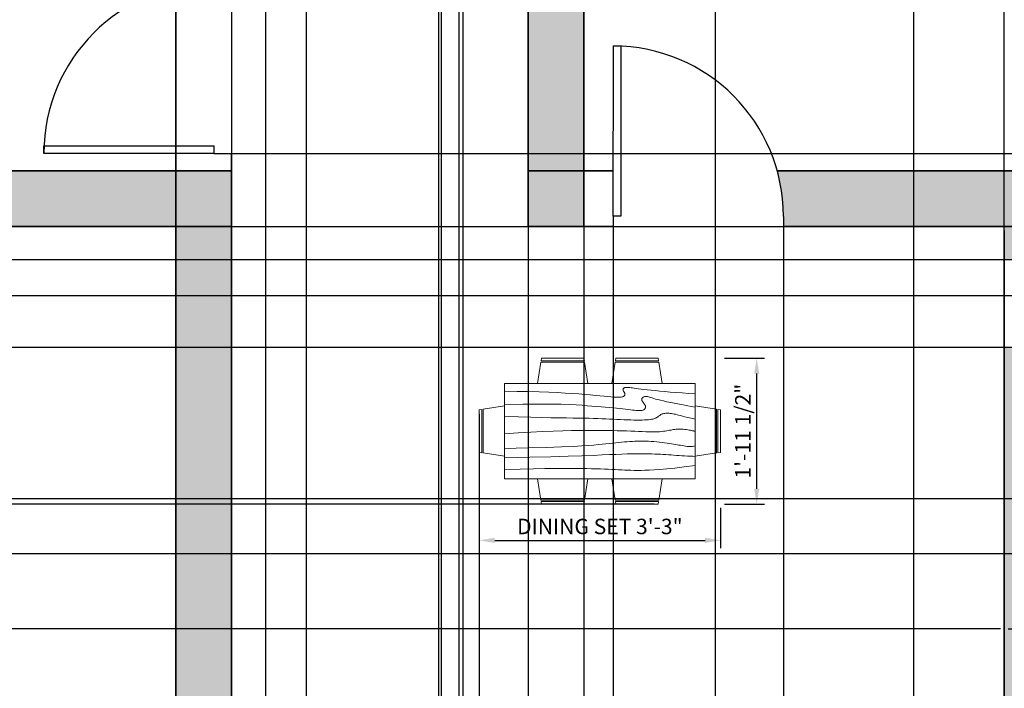
# Model space of a CAD drawing. Units: millimetres. Extents: x 2856 to 3283, y 634 to 1474.
# Tile 6 of 8: x 3006 to 3165, y 1213 to 1321. Entities that reach past the tile are written whole.
import ezdxf

# ---------------------------------------------------------------- set-up
doc = ezdxf.new("R2010")
doc.units = ezdxf.units.MM
for name, color, linetype, lineweight in [('A-ANNO-DIMS', 90, 'Continuous', 18), ('A-WALL-PATT', 2, 'Continuous', 13), ('doors', 10, 'Continuous', 25), ('furniture', 140, 'Continuous', 18), ('walls', 50, 'Continuous', 35)]:
    doc.layers.add(name, color=color, linetype=linetype, lineweight=lineweight)
doc.styles.get("Standard").update_dxf_attribs({"font": 'arial.ttf'})
doc.dimstyles.new('ISO-25', dxfattribs={"dimtxt": 2.5, "dimasz": 2.5, "dimexe": 1.25, "dimexo": 0.625, "dimtad": 1, "dimdec": 0, "dimlunit": 3, "dimtxsty": 'Standard', "dimcen": 2.5, "dimadec": 0, "dimazin": 0, "dimtfac": 1, "dimtdec": 0, "dimtmove": 0, "dimatfit": 3, "dimfxl": 1, "dimarcsym": 0})

# ---------------------------------------------------------------- blocks, each defined once
blk = doc.blocks.new('*U3')
for p, q in [((0, 0), (0, -6)), ((40, 0), (40, -6))]:
    blk.add_line(p, q)
blk.add_lwpolyline([(0, 0), (0, 40), (1.75, 40), (1.75, 0)], close=True)
blk.add_arc((0, 0), 40, 0, 90)
blk = doc.blocks.new('Dining Set - 36 x 72 in.')
for p, q in [((-22.2343, 26.00059), (-23.4847, 17.99762)), ((-22.2304, 26), (-5.7608, 26)), ((-22, 27.5), (-22.1562, 26.50042)), ((-5.8416, 26.5), (-22.1534, 26.5)), ((-22, 27.5), (-6, 27.5)), ((-5.8437, 26.49966), (-6, 27.5)), ((-4.5152, 17.99762), (-5.7655, 25.99926)), ((5.7657, 26.00059), (4.5153, 17.99762)), ((5.7696, 26), (22.2392, 26)), ((6, 27.5), (5.8438, 26.50042)), ((22.1584, 26.5), (5.8466, 26.5)), ((6, 27.5), (22, 27.5)), ((22.1563, 26.49966), (22, 27.5)), ((23.4848, 17.99762), (22.2345, 25.99926)), ((36, 18), (-36, 18)), ((-36, 18), (-36, -18)), ((36, -18), (36, 18)), ((-45.5, 8), (-44.5004, 8.15617)), ((-45.5, 8), (-45.5, -8)), ((-44.5, -8.15843), (-44.5, 8.15338)), ((-44.0006, 8.23428), (-35.9976, 9.48474)), ((-44, 8.23041), (-44, -8.23915)), ((44.0006, 8.23428), (35.9976, 9.48474)), ((44, 8.23041), (44, -8.23915)), ((44.5, -8.15843), (44.5, 8.15338)), ((45.5, 8), (44.5005, 8.15617)), ((45.5, 8), (45.5, -8)), ((-44.4997, -8.15631), (-45.5, -8)), ((-35.9976, -9.48476), (-43.9993, -8.2345)), ((35.9976, -9.48476), (43.9993, -8.2345)), ((44.4997, -8.15631), (45.5, -8)), ((-36, -18), (36, -18)), ((-22.2343, -26.0006), (-23.4847, -17.99762)), ((-4.5152, -17.99762), (-5.7655, -25.99928)), ((5.7657, -26.0006), (4.5153, -17.99762)), ((23.4848, -17.99762), (22.2345, -25.99928)), ((-22.2304, -26), (-5.7608, -26)), ((-22, -27.5), (-22.1562, -26.50044)), ((-5.8416, -26.5), (-22.1534, -26.5)), ((-22, -27.5), (-6, -27.5)), ((-5.8437, -26.49967), (-6, -27.5)), ((5.7696, -26), (22.2392, -26)), ((6, -27.5), (5.8438, -26.50044)), ((22.1584, -26.5), (5.8466, -26.5)), ((6, -27.5), (22, -27.5)), ((22.1563, -26.49967), (22, -27.5))]:
    blk.add_line(p, q)
for points in [[(-36, 15), (-31.1772, 14.97754), (-26.8079, 14.91406), (-22.8538, 14.81543), (-19.276, 14.6875), (-16.0362, 14.53613), (-13.0957, 14.36718), (-10.4159, 14.18652), (-7.9583, 14), (-5.6904, 13.81315), (-3.6035, 13.63021), (-1.6954, 13.45508), (0.0365, 13.29166), (1.5945, 13.14388), (2.9811, 13.01562), (4.1988, 12.9108), (5.25, 12.83333), (6.1393, 12.78613), (6.8802, 12.76823), (7.4883, 12.77767), (7.9792, 12.8125), (8.3685, 12.87077), (8.6719, 12.95052), (8.9049, 13.0498), (9.0833, 13.16666), (9.2205, 13.29899), (9.3216, 13.44401), (9.3895, 13.59879), (9.4271, 13.76041), (9.4373, 13.92594), (9.4232, 14.09245), (9.3875, 14.257), (9.3333, 14.41666), (9.2638, 14.56917), (9.1836, 14.71484), (9.0975, 14.85465), (9.0104, 14.98958), (8.9272, 15.1206), (8.8529, 15.2487), (8.7922, 15.37483), (8.75, 15.5), (8.7305, 15.62467), (8.7344, 15.74739), (8.7617, 15.86621), (8.8125, 15.97916), (8.8867, 16.08431), (8.9844, 16.17968), (9.1055, 16.26334), (9.25, 16.33333), (9.4189, 16.38802), (9.6172, 16.42708), (9.8506, 16.45052), (10.125, 16.45833), (10.4463, 16.45052), (10.8203, 16.42708), (11.2529, 16.38802), (11.75, 16.33333), (12.3184, 16.26318), (12.9694, 16.17838), (13.7151, 16.07991), (14.5677, 15.96875), (15.5395, 15.84586), (16.6426, 15.71224), (17.8893, 15.56884), (19.2917, 15.41666), (20.859, 15.25667), (22.5879, 15.08984), (24.4721, 14.91715), (26.5052, 14.73958), (28.6809, 14.5581), (30.9929, 14.3737), (33.4347, 14.18733), (36, 14)], [(-36, 10), (-28.9766, 10.14274), (-23.1725, 10.20442), (-18.4241, 10.19775), (-14.5677, 10.13541), (-11.4399, 10.03011), (-8.877, 9.89453), (-6.7154, 9.74137), (-4.7917, 9.58333), (-2.9698, 9.43082), (-1.2246, 9.28515), (0.4415, 9.14534), (2.026, 9.01041), (3.5266, 8.87939), (4.9408, 8.7513), (6.266, 8.62516), (7.5, 8.5), (8.6411, 8.37549), (9.6914, 8.2539), (10.6538, 8.13818), (11.5312, 8.03125), (12.3267, 7.93603), (13.043, 7.85547), (13.6831, 7.79248), (14.25, 7.75), (14.7471, 7.7303), (15.1797, 7.73307), (15.5537, 7.75732), (15.875, 7.80208), (16.1494, 7.86637), (16.3828, 7.94922), (16.5811, 8.04964), (16.75, 8.16666), (16.8944, 8.29915), (17.0143, 8.44531), (17.1089, 8.60319), (17.1771, 8.77083), (17.218, 8.94629), (17.2305, 9.1276), (17.2137, 9.31282), (17.1667, 9.5), (17.0895, 9.6875), (16.987, 9.875), (16.8649, 10.0625), (16.7292, 10.25), (16.5856, 10.4375), (16.4401, 10.625), (16.2985, 10.8125), (16.1667, 11), (16.05, 11.18733), (15.9518, 11.3737), (15.8752, 11.5581), (15.8229, 11.73958), (15.798, 11.91715), (15.8034, 12.08984), (15.842, 12.25667), (15.9167, 12.41666), (16.0295, 12.56836), (16.1784, 12.70833), (16.3605, 12.83268), (16.5729, 12.9375), (16.8127, 13.01888), (17.0768, 13.07291), (17.3625, 13.0957), (17.6667, 13.08333), (17.9894, 13.03312), (18.3418, 12.94726), (18.7382, 12.82918), (19.1927, 12.68229), (19.7195, 12.51001), (20.3327, 12.31575), (21.0465, 12.10294), (21.875, 11.875), (22.8357, 11.63354), (23.959, 11.37304), (25.2786, 11.08618), (26.8282, 10.76562), (28.6414, 10.40405), (30.752, 9.99414), (33.1936, 9.52856), (36, 9)], [(-36, 5.5), (-30.7157, 5.3348), (-26.069, 5.20963), (-21.9946, 5.11767), (-18.4271, 5.05208), (-15.3009, 5.00602), (-12.5508, 4.97265), (-10.1112, 4.94515), (-7.9167, 4.91666), (-5.909, 4.88167), (-4.0586, 4.83984), (-2.3429, 4.79215), (-0.7396, 4.73958), (0.7739, 4.6831), (2.22, 4.6237), (3.6213, 4.56233), (5, 4.5), (6.373, 4.43782), (7.7344, 4.3776), (9.0723, 4.32129), (10.375, 4.27083), (11.6309, 4.22819), (12.8281, 4.19531), (13.9551, 4.17415), (15, 4.16666), (15.954, 4.17448), (16.819, 4.19791), (17.6001, 4.23698), (18.3021, 4.29166), (18.9299, 4.36198), (19.4883, 4.44791), (19.9823, 4.54948), (20.4167, 4.66666), (20.7969, 4.79899), (21.1302, 4.94401), (21.4245, 5.09879), (21.6875, 5.26041), (21.9271, 5.42594), (22.1511, 5.59245), (22.3672, 5.757), (22.5834, 5.91666), (22.8065, 6.06868), (23.0404, 6.21093), (23.2879, 6.34147), (23.5521, 6.45833), (23.8358, 6.55957), (24.142, 6.64323), (24.4735, 6.70735), (24.8334, 6.75), (25.2235, 6.76969), (25.642, 6.76692), (26.0858, 6.74267), (26.5521, 6.69791), (27.0379, 6.63362), (27.5404, 6.55078), (28.0565, 6.45036), (28.5834, 6.33333), (29.1242, 6.19987), (29.7071, 6.04687), (30.3661, 5.87044), (31.1354, 5.66666), (32.0493, 5.43164), (33.142, 5.16146), (34.4475, 4.85221), (36, 4.5)], [(-36, -1), (-30.7915, -0.6591), (-26.0195, -0.38216), (-21.6519, -0.16284), (-17.6563, 0.00521), (-14.0005, 0.12833), (-10.6523, 0.21289), (-7.5796, 0.26522), (-4.75, 0.29166), (-2.134, 0.29793), (0.2878, 0.28711), (2.5317, 0.26163), (4.6146, 0.22396), (6.5529, 0.17651), (8.3633, 0.12174), (10.0623, 0.06209), (11.6667, 0), (13.1899, -0.06201), (14.6341, -0.1211), (15.9982, -0.17432), (17.2813, -0.21875), (18.4823, -0.25147), (19.6003, -0.26953), (20.6343, -0.27002), (21.5834, -0.25), (22.4481, -0.20768), (23.2357, -0.14584), (23.9549, -0.06836), (24.6146, 0.02083), (25.2235, 0.11784), (25.7904, 0.21875), (26.3241, 0.31966), (26.8334, 0.41666), (27.3265, 0.50618), (27.8099, 0.58593), (28.2894, 0.65397), (28.7709, 0.70833), (29.2601, 0.74707), (29.763, 0.76823), (30.2855, 0.76985), (30.8334, 0.75), (31.4088, 0.70784), (31.9994, 0.64713), (32.589, 0.57275), (33.1615, 0.48958), (33.7008, 0.4025), (34.1908, 0.3164), (34.6153, 0.23616), (34.9584, 0.16666), (35.2099, 0.11165), (35.3848, 0.07031), (35.504, 0.04069), (35.5886, 0.02083), (35.6594, 0.00879), (35.7377, 0.0026), (35.8442, 0.00032), (36, 0)], [(-36, -6.5), (-27.1843, -6.31267), (-20.084, -6.1263), (-14.469, -5.9419), (-10.1094, -5.76042), (-6.7752, -5.58285), (-4.2363, -5.41016), (-2.2629, -5.24333), (-0.625, -5.08334), (0.8708, -4.93099), (2.2715, -4.78646), (3.5872, -4.64974), (4.8281, -4.52084), (6.0046, -4.39974), (7.127, -4.28646), (8.2053, -4.18099), (9.25, -4.08334), (10.2705, -3.99382), (11.2734, -3.91407), (12.2647, -3.84603), (13.25, -3.79167), (14.2354, -3.75293), (15.2266, -3.73177), (16.2295, -3.73015), (17.25, -3.75), (18.2912, -3.79248), (19.3451, -3.85547), (20.4009, -3.93604), (21.4479, -4.03125), (22.4754, -4.13819), (23.4727, -4.25391), (24.4289, -4.37549), (25.3334, -4.5), (26.1785, -4.62492), (26.9694, -4.74935), (27.7145, -4.87281), (28.4219, -4.99479), (29.1, -5.11483), (29.7572, -5.23242), (30.4016, -5.34709), (31.0417, -5.45834), (31.6837, -5.56437), (32.3262, -5.65821), (32.9658, -5.73153), (33.599, -5.77604), (34.2224, -5.78345), (34.8327, -5.74545), (35.4264, -5.65373), (36, -5.5)], [(-36, -10), (-26.4022, -9.81299), (-18.4675, -9.62891), (-11.9839, -9.45069), (-6.7396, -9.28125), (-2.5226, -9.12354), (0.8789, -8.98047), (3.6769, -8.85498), (6.0833, -8.75), (8.2767, -8.66765), (10.3021, -8.60677), (12.1712, -8.56543), (13.8958, -8.54167), (15.4876, -8.53353), (16.9583, -8.53907), (18.3197, -8.55632), (19.5834, -8.58334), (20.7616, -8.61841), (21.8685, -8.66081), (22.9188, -8.71004), (23.9271, -8.76563), (24.9081, -8.82707), (25.8763, -8.89388), (26.8465, -8.96558), (27.8334, -9.04167), (28.8474, -9.12118), (29.8828, -9.20117), (30.93, -9.27824), (31.9792, -9.34896), (33.0205, -9.40991), (34.0443, -9.45768), (35.0407, -9.48885), (36, -9.5)], [(-36, -14.5), (-30.0881, -14.33513), (-25.0332, -14.21224), (-20.7312, -14.12647), (-17.0781, -14.07292), (-13.97, -14.04671), (-11.3027, -14.04297), (-8.9724, -14.05681), (-6.875, -14.08334), (-4.9224, -14.11833), (-3.0905, -14.16016), (-1.3709, -14.20785), (0.2448, -14.26042), (1.7647, -14.3169), (3.1973, -14.3763), (4.5507, -14.43767), (5.8333, -14.5), (7.0554, -14.5621), (8.235, -14.62175), (9.3922, -14.67652), (10.5469, -14.72396), (11.7192, -14.76164), (12.929, -14.78711), (14.1965, -14.79794), (15.5417, -14.79167), (16.9933, -14.76424), (18.6152, -14.70508), (20.4804, -14.60197), (22.6615, -14.44271), (25.2312, -14.21509), (28.2624, -13.9069), (31.8277, -13.50594), (36, -13)]]:
    blk.add_lwpolyline(points)
blk = doc.blocks.new('*D26')
at = {"layer": 'A-ANNO-DIMS', "color": 0, "lineweight": -2, "transparency": 16777216}
for p, q in [((3080.25, 1242.47), (3080.25, 1235.99)), ((3119.28, 1242.47), (3119.28, 1235.99)), ((3082.75, 1237.24), (3116.78, 1237.24))]:
    blk.add_line(p, q, dxfattribs=at)
at = {"layer": 'A-ANNO-DIMS', "color": 0, "transparency": 16777216}
for points in [[(3082.75, 1237.66), (3082.75, 1236.82), (3080.25, 1237.24)], [(3116.78, 1237.66), (3116.78, 1236.82), (3119.28, 1237.24)]]:
    blk.add_solid(points, dxfattribs=at)
at = {"layer": 'Defpoints', "color": 0, "transparency": 16777216}
for p in [(3080.25, 1243.09), (3119.28, 1243.09), (3119.28, 1237.24)]:
    blk.add_point(p, dxfattribs=at)
at = {"layer": 'A-ANNO-DIMS', "color": 0, "transparency": 16777216, "insert": (3099.76, 1239.16), "char_height": 2.5, "attachment_point": 5}
blk.add_mtext('DINING SET 3\'-3"', dxfattribs=at)
blk = doc.blocks.new('*D27')
at = {"layer": 'A-ANNO-DIMS', "color": 0, "lineweight": -2, "transparency": 16777216}
for p, q in [((3119.9, 1266.68), (3126.38, 1266.68)), ((3125.13, 1245.59), (3125.13, 1264.18)), ((3119.9, 1243.09), (3126.38, 1243.09))]:
    blk.add_line(p, q, dxfattribs=at)
at = {"layer": 'A-ANNO-DIMS', "color": 0, "transparency": 16777216}
for points in [[(3124.72, 1264.18), (3125.55, 1264.18), (3125.13, 1266.68)], [(3124.72, 1245.59), (3125.55, 1245.59), (3125.13, 1243.09)]]:
    blk.add_solid(points, dxfattribs=at)
at = {"layer": 'Defpoints', "color": 0, "transparency": 16777216}
for p in [(3119.28, 1266.68), (3125.13, 1266.68), (3119.28, 1243.09)]:
    blk.add_point(p, dxfattribs=at)
at = {"layer": 'A-ANNO-DIMS', "color": 0, "transparency": 16777216, "insert": (3123.21, 1254.89), "char_height": 2.5, "attachment_point": 5, "rotation": 90}
blk.add_mtext('1\'-11 1/2"', dxfattribs=at)
blk = doc.blocks.new('*D33')
at = {"layer": 'A-ANNO-DIMS', "color": 0, "lineweight": -2, "transparency": 16777216}
for p, q in [((3073.7, 1014.05), (3073.7, 1470.06)), ((3224.18, 1014.05), (3224.18, 1470.06)), ((3076.2, 1468.81), (3221.68, 1468.81))]:
    blk.add_line(p, q, dxfattribs=at)
at = {"layer": 'A-ANNO-DIMS', "color": 0, "transparency": 16777216}
for points in [[(3076.2, 1469.23), (3076.2, 1468.4), (3073.7, 1468.81)], [(3221.68, 1469.23), (3221.68, 1468.4), (3224.18, 1468.81)]]:
    blk.add_solid(points, dxfattribs=at)
at = {"layer": 'Defpoints', "color": 0, "transparency": 16777216}
for p in [(3224.18, 1468.81), (3073.7, 1013.42), (3224.18, 1013.42)]:
    blk.add_point(p, dxfattribs=at)
at = {"layer": 'A-ANNO-DIMS', "color": 0, "transparency": 16777216, "insert": (3148.94, 1470.73), "char_height": 2.5, "attachment_point": 5}
blk.add_mtext('12\'-6 1/2"', dxfattribs=at)
blk = doc.blocks.new('*D40')
at = {"layer": 'A-ANNO-DIMS', "color": 0, "lineweight": -2, "transparency": 16777216}
for p, q in [((3118.44, 913.07), (3118.44, 1470.06)), ((3174.82, 914.65), (3174.82, 1470.06)), ((3120.94, 1468.81), (3172.32, 1468.81))]:
    blk.add_line(p, q, dxfattribs=at)
at = {"layer": 'A-ANNO-DIMS', "color": 0, "transparency": 16777216}
for points in [[(3120.94, 1469.23), (3120.94, 1468.4), (3118.44, 1468.81)], [(3172.32, 1469.23), (3172.32, 1468.4), (3174.82, 1468.81)]]:
    blk.add_solid(points, dxfattribs=at)
at = {"layer": 'Defpoints', "color": 0, "transparency": 16777216}
for p in [(3174.82, 1468.81), (3174.82, 914.03), (3118.44, 912.44)]:
    blk.add_point(p, dxfattribs=at)
at = {"layer": 'A-ANNO-DIMS', "color": 0, "transparency": 16777216, "insert": (3146.63, 1470.73), "char_height": 2.5, "attachment_point": 5}
blk.add_mtext('4\'-8 1/2"', dxfattribs=at)
blk = doc.blocks.new('*D43')
at = {"layer": 'A-ANNO-DIMS', "color": 0, "lineweight": -2, "transparency": 16777216}
for p, q in [((3052.34, 800.56), (3052.34, 1470.06)), ((3077.68, 819.72), (3077.68, 1470.06)), ((3054.84, 1468.81), (3075.18, 1468.81))]:
    blk.add_line(p, q, dxfattribs=at)
at = {"layer": 'A-ANNO-DIMS', "color": 0, "transparency": 16777216}
for points in [[(3054.84, 1469.23), (3054.84, 1468.4), (3052.34, 1468.81)], [(3075.18, 1469.23), (3075.18, 1468.4), (3077.68, 1468.81)]]:
    blk.add_solid(points, dxfattribs=at)
at = {"layer": 'Defpoints', "color": 0, "transparency": 16777216}
for p in [(3077.68, 1468.81), (3077.68, 819.09), (3052.34, 799.94)]:
    blk.add_point(p, dxfattribs=at)
at = {"layer": 'A-ANNO-DIMS', "color": 0, "transparency": 16777216, "insert": (3065.01, 1470.73), "char_height": 2.5, "attachment_point": 5}
blk.add_mtext('2\'-1 1/2"', dxfattribs=at)
blk = doc.blocks.new('*D50')
at = {"layer": 'A-ANNO-DIMS', "color": 0, "lineweight": -2, "transparency": 16777216}
for p, q in [((3031.17, 1166.56), (3031.17, 1470.06)), ((3165.17, 1157.56), (3165.17, 1470.06)), ((3033.67, 1468.81), (3162.67, 1468.81))]:
    blk.add_line(p, q, dxfattribs=at)
at = {"layer": 'A-ANNO-DIMS', "color": 0, "transparency": 16777216}
for points in [[(3033.67, 1469.23), (3033.67, 1468.4), (3031.17, 1468.81)], [(3162.67, 1469.23), (3162.67, 1468.4), (3165.17, 1468.81)]]:
    blk.add_solid(points, dxfattribs=at)
at = {"layer": 'Defpoints', "color": 0, "transparency": 16777216}
for p in [(3165.17, 1468.81), (3031.17, 1165.94), (3165.17, 1156.94)]:
    blk.add_point(p, dxfattribs=at)
at = {"layer": 'A-ANNO-DIMS', "color": 0, "transparency": 16777216, "insert": (3098.17, 1470.69), "char_height": 2.5, "attachment_point": 5}
blk.add_mtext('11\'-2"', dxfattribs=at)
blk = doc.blocks.new('*D51')
at = {"layer": 'A-ANNO-DIMS', "color": 0, "lineweight": -2, "transparency": 16777216}
for p, q in [((3165.17, 1223.56), (3165.17, 1470.06)), ((3243.17, 1223.56), (3243.17, 1470.06)), ((3167.67, 1468.81), (3240.67, 1468.81))]:
    blk.add_line(p, q, dxfattribs=at)
at = {"layer": 'A-ANNO-DIMS', "color": 0, "transparency": 16777216}
for points in [[(3167.67, 1469.23), (3167.67, 1468.4), (3165.17, 1468.81)], [(3240.67, 1469.23), (3240.67, 1468.4), (3243.17, 1468.81)]]:
    blk.add_solid(points, dxfattribs=at)
at = {"layer": 'Defpoints', "color": 0, "transparency": 16777216}
for p in [(3243.17, 1468.81), (3165.17, 1222.94), (3243.17, 1222.94)]:
    blk.add_point(p, dxfattribs=at)
at = {"layer": 'A-ANNO-DIMS', "color": 0, "transparency": 16777216, "insert": (3204.17, 1470.71), "char_height": 2.5, "attachment_point": 5}
blk.add_mtext('6\'-6"', dxfattribs=at)
blk = doc.blocks.new('*D59')
at = {"layer": 'A-ANNO-DIMS', "color": 0, "lineweight": -2, "transparency": 16777216}
for p, q in [((2959.17, 1117.56), (2959.17, 1470.06)), ((3074.17, 1117.56), (3074.17, 1470.06)), ((2961.67, 1468.81), (3071.67, 1468.81))]:
    blk.add_line(p, q, dxfattribs=at)
at = {"layer": 'A-ANNO-DIMS', "color": 0, "transparency": 16777216}
for points in [[(2961.67, 1469.23), (2961.67, 1468.4), (2959.17, 1468.81)], [(3071.67, 1469.23), (3071.67, 1468.4), (3074.17, 1468.81)]]:
    blk.add_solid(points, dxfattribs=at)
at = {"layer": 'Defpoints', "color": 0, "transparency": 16777216}
for p in [(3074.17, 1468.81), (2959.17, 1116.94), (3074.17, 1116.94)]:
    blk.add_point(p, dxfattribs=at)
at = {"layer": 'A-ANNO-DIMS', "color": 0, "transparency": 16777216, "insert": (3016.67, 1470.71), "char_height": 2.5, "attachment_point": 5}
blk.add_mtext('9\'-7"', dxfattribs=at)
blk = doc.blocks.new('*D61')
at = {"layer": 'A-ANNO-DIMS', "color": 0, "lineweight": -2, "transparency": 16777216}
for p, q in [((3031.17, 1430.31), (3031.17, 634.81)), ((3040.17, 1430.31), (3040.17, 634.81)), ((3033.67, 636.06), (3037.67, 636.06))]:
    blk.add_line(p, q, dxfattribs=at)
at = {"layer": 'A-ANNO-DIMS', "color": 0, "transparency": 16777216}
for points in [[(3033.67, 636.48), (3033.67, 635.65), (3031.17, 636.06)], [(3037.67, 636.48), (3037.67, 635.65), (3040.17, 636.06)]]:
    blk.add_solid(points, dxfattribs=at)
at = {"layer": 'Defpoints', "color": 0, "transparency": 16777216}
for p in [(3031.17, 1430.94), (3040.17, 1430.94), (3040.17, 636.06)]:
    blk.add_point(p, dxfattribs=at)
at = {"layer": 'A-ANNO-DIMS', "color": 0, "transparency": 16777216, "insert": (3035.67, 637.96), "char_height": 2.5, "attachment_point": 5}
blk.add_mtext('0\'-9"', dxfattribs=at)
blk = doc.blocks.new('*D62')
at = {"layer": 'A-ANNO-DIMS', "color": 0, "lineweight": -2, "transparency": 16777216}
for p, q in [((3101.93, 1287.31), (3101.93, 634.81)), ((3129.44, 1287.31), (3129.44, 634.81)), ((3104.43, 636.06), (3126.94, 636.06))]:
    blk.add_line(p, q, dxfattribs=at)
at = {"layer": 'A-ANNO-DIMS', "color": 0, "transparency": 16777216}
for points in [[(3104.43, 636.48), (3104.43, 635.65), (3101.93, 636.06)], [(3126.94, 636.48), (3126.94, 635.65), (3129.44, 636.06)]]:
    blk.add_solid(points, dxfattribs=at)
at = {"layer": 'Defpoints', "color": 0, "transparency": 16777216}
for p in [(3101.93, 1287.94), (3129.44, 1287.94), (3129.44, 636.06)]:
    blk.add_point(p, dxfattribs=at)
at = {"layer": 'A-ANNO-DIMS', "color": 0, "transparency": 16777216, "insert": (3115.68, 637.98), "char_height": 2.5, "attachment_point": 5}
blk.add_mtext('2\'-3 1/2"', dxfattribs=at)
blk = doc.blocks.new('*D63')
at = {"layer": 'A-ANNO-DIMS', "color": 0, "lineweight": -2, "transparency": 16777216}
for p, q in [((3164.55, 1282.56), (2860.05, 1282.56)), ((2861.3, 1270.93), (2861.3, 1280.06)), ((3164.55, 1268.43), (2860.05, 1268.43))]:
    blk.add_line(p, q, dxfattribs=at)
at = {"layer": 'A-ANNO-DIMS', "color": 0, "transparency": 16777216}
for points in [[(2860.88, 1280.06), (2861.72, 1280.06), (2861.3, 1282.56)], [(2860.88, 1270.93), (2861.72, 1270.93), (2861.3, 1268.43)]]:
    blk.add_solid(points, dxfattribs=at)
at = {"layer": 'Defpoints', "color": 0, "transparency": 16777216}
for p in [(2861.3, 1282.56), (3165.17, 1282.56), (3165.17, 1268.43)]:
    blk.add_point(p, dxfattribs=at)
at = {"layer": 'A-ANNO-DIMS', "color": 0, "transparency": 16777216, "insert": (2859.42, 1275.5), "char_height": 2.5, "attachment_point": 5, "rotation": 90}
blk.add_mtext('1\'-2"', dxfattribs=at)
blk = doc.blocks.new('*D68')
at = {"layer": 'A-ANNO-DIMS', "color": 0, "lineweight": -2, "transparency": 16777216}
for p, q in [((3040.8, 1327.29), (3282.3, 1327.29)), ((3281.05, 1302.28), (3281.05, 1324.79)), ((3040.8, 1299.78), (3282.3, 1299.78))]:
    blk.add_line(p, q, dxfattribs=at)
at = {"layer": 'A-ANNO-DIMS', "color": 0, "transparency": 16777216}
for points in [[(3280.63, 1324.79), (3281.47, 1324.79), (3281.05, 1327.29)], [(3280.63, 1302.28), (3281.47, 1302.28), (3281.05, 1299.78)]]:
    blk.add_solid(points, dxfattribs=at)
at = {"layer": 'Defpoints', "color": 0, "transparency": 16777216}
for p in [(3040.17, 1327.29), (3281.05, 1327.29), (3040.17, 1299.78)]:
    blk.add_point(p, dxfattribs=at)
at = {"layer": 'A-ANNO-DIMS', "color": 0, "transparency": 16777216, "insert": (3279.13, 1313.53), "char_height": 2.5, "attachment_point": 5, "rotation": 90}
blk.add_mtext('2\'-3 1/2"', dxfattribs=at)
blk = doc.blocks.new('*D70')
at = {"layer": 'A-ANNO-DIMS', "color": 0, "lineweight": -2, "transparency": 16777216}
for p, q in [((3045.69, 1421.31), (3045.69, 634.81)), ((3076.97, 1421.31), (3076.97, 634.81)), ((3048.19, 636.06), (3074.47, 636.06))]:
    blk.add_line(p, q, dxfattribs=at)
at = {"layer": 'A-ANNO-DIMS', "color": 0, "transparency": 16777216}
for points in [[(3048.19, 636.48), (3048.19, 635.65), (3045.69, 636.06)], [(3074.47, 636.48), (3074.47, 635.65), (3076.97, 636.06)]]:
    blk.add_solid(points, dxfattribs=at)
at = {"layer": 'Defpoints', "color": 0, "transparency": 16777216}
for p in [(3045.69, 1421.94), (3076.97, 1421.94), (3076.97, 636.06)]:
    blk.add_point(p, dxfattribs=at)
at = {"layer": 'A-ANNO-DIMS', "color": 0, "transparency": 16777216, "insert": (3061.33, 637.98), "char_height": 2.5, "attachment_point": 5}
blk.add_mtext('2\'-7 1/2"', dxfattribs=at)
blk = doc.blocks.new('*D71')
at = {"layer": 'A-ANNO-DIMS', "color": 0, "lineweight": -2, "transparency": 16777216}
for p, q in [((3150.5, 1421.31), (3150.5, 634.81)), ((3189.65, 1421.31), (3189.65, 634.81)), ((3153, 636.06), (3187.15, 636.06))]:
    blk.add_line(p, q, dxfattribs=at)
at = {"layer": 'A-ANNO-DIMS', "color": 0, "transparency": 16777216}
for points in [[(3153, 636.48), (3153, 635.65), (3150.5, 636.06)], [(3187.15, 636.48), (3187.15, 635.65), (3189.65, 636.06)]]:
    blk.add_solid(points, dxfattribs=at)
at = {"layer": 'Defpoints', "color": 0, "transparency": 16777216}
for p in [(3150.5, 1421.94), (3189.65, 1421.94), (3189.65, 636.06)]:
    blk.add_point(p, dxfattribs=at)
at = {"layer": 'A-ANNO-DIMS', "color": 0, "transparency": 16777216, "insert": (3170.07, 637.97), "char_height": 2.5, "attachment_point": 5}
blk.add_mtext('3\'-3"', dxfattribs=at)
blk = doc.blocks.new('*D73')
at = {"layer": 'A-ANNO-DIMS', "color": 0, "lineweight": -2, "transparency": 16777216}
for p, q in [((2908.8, 1235.12), (3282.3, 1235.12)), ((3281.05, 1193.19), (3281.05, 1232.62)), ((2908.8, 1190.69), (3282.3, 1190.69))]:
    blk.add_line(p, q, dxfattribs=at)
at = {"layer": 'A-ANNO-DIMS', "color": 0, "transparency": 16777216}
for points in [[(3280.63, 1232.62), (3281.47, 1232.62), (3281.05, 1235.12)], [(3280.63, 1193.19), (3281.47, 1193.19), (3281.05, 1190.69)]]:
    blk.add_solid(points, dxfattribs=at)
at = {"layer": 'Defpoints', "color": 0, "transparency": 16777216}
for p in [(2908.17, 1235.12), (3281.05, 1235.12), (2908.17, 1190.69)]:
    blk.add_point(p, dxfattribs=at)
at = {"layer": 'A-ANNO-DIMS', "color": 0, "transparency": 16777216, "insert": (3279.13, 1212.91), "char_height": 2.5, "attachment_point": 5, "rotation": 90}
blk.add_mtext('3\'-8 1/2"', dxfattribs=at)
blk = doc.blocks.new('*D74')
at = {"layer": 'A-ANNO-DIMS', "color": 0, "lineweight": -2, "transparency": 16777216}
for p, q in [((3233.55, 1276.76), (2860.05, 1276.76)), ((2861.3, 1246.44), (2861.3, 1274.26)), ((3233.55, 1243.94), (2860.05, 1243.94))]:
    blk.add_line(p, q, dxfattribs=at)
at = {"layer": 'A-ANNO-DIMS', "color": 0, "transparency": 16777216}
for points in [[(2860.88, 1274.26), (2861.72, 1274.26), (2861.3, 1276.76)], [(2860.88, 1246.44), (2861.72, 1246.44), (2861.3, 1243.94)]]:
    blk.add_solid(points, dxfattribs=at)
at = {"layer": 'Defpoints', "color": 0, "transparency": 16777216}
for p in [(2861.3, 1276.76), (3234.17, 1276.76), (3234.17, 1243.94)]:
    blk.add_point(p, dxfattribs=at)
at = {"layer": 'A-ANNO-DIMS', "color": 0, "transparency": 16777216, "insert": (2859.4, 1260.35), "char_height": 2.5, "attachment_point": 5, "rotation": 90}
blk.add_mtext('2\'-9"', dxfattribs=at)
blk = doc.blocks.new('*D77')
at = {"layer": 'A-ANNO-DIMS', "color": 0, "lineweight": -2, "transparency": 16777216}
for p, q in [((3097.17, 1430.31), (3097.17, 634.81)), ((3150.5, 1421.31), (3150.5, 634.81)), ((3099.67, 636.06), (3148, 636.06))]:
    blk.add_line(p, q, dxfattribs=at)
at = {"layer": 'A-ANNO-DIMS', "color": 0, "transparency": 16777216}
for points in [[(3099.67, 636.48), (3099.67, 635.65), (3097.17, 636.06)], [(3148, 636.48), (3148, 635.65), (3150.5, 636.06)]]:
    blk.add_solid(points, dxfattribs=at)
at = {"layer": 'Defpoints', "color": 0, "transparency": 16777216}
for p in [(3097.17, 1430.94), (3150.5, 1421.94), (3150.5, 636.06)]:
    blk.add_point(p, dxfattribs=at)
at = {"layer": 'A-ANNO-DIMS', "color": 0, "transparency": 16777216, "insert": (3123.84, 637.98), "char_height": 2.5, "attachment_point": 5}
blk.add_mtext('4\'-5 1/2"', dxfattribs=at)
blk = doc.blocks.new('*D79')
at = {"layer": 'A-ANNO-DIMS', "color": 0, "lineweight": -2, "transparency": 16777216}
for p, q in [((2899.8, 1287.94), (3282.3, 1287.94)), ((3281.05, 1237.62), (3281.05, 1285.44)), ((2908.8, 1235.12), (3282.3, 1235.12))]:
    blk.add_line(p, q, dxfattribs=at)
at = {"layer": 'A-ANNO-DIMS', "color": 0, "transparency": 16777216}
for points in [[(3280.63, 1285.44), (3281.47, 1285.44), (3281.05, 1287.94)], [(3280.63, 1237.62), (3281.47, 1237.62), (3281.05, 1235.12)]]:
    blk.add_solid(points, dxfattribs=at)
at = {"layer": 'Defpoints', "color": 0, "transparency": 16777216}
for p in [(2899.17, 1287.94), (3281.05, 1287.94), (2908.17, 1235.12)]:
    blk.add_point(p, dxfattribs=at)
at = {"layer": 'A-ANNO-DIMS', "color": 0, "transparency": 16777216, "insert": (3279.15, 1261.53), "char_height": 2.5, "attachment_point": 5, "rotation": 90}
blk.add_mtext('4\'-5"', dxfattribs=at)
blk = doc.blocks.new('*D81')
at = {"layer": 'A-ANNO-DIMS', "color": 0, "lineweight": -2, "transparency": 16777216}
for p, q in [((3174.8, 1240.31), (3282.3, 1240.31)), ((3281.05, 1225.44), (3281.05, 1237.81)), ((3165.8, 1222.94), (3282.3, 1222.94))]:
    blk.add_line(p, q, dxfattribs=at)
at = {"layer": 'A-ANNO-DIMS', "color": 0, "transparency": 16777216}
for points in [[(3280.63, 1237.81), (3281.47, 1237.81), (3281.05, 1240.31)], [(3280.63, 1225.44), (3281.47, 1225.44), (3281.05, 1222.94)]]:
    blk.add_solid(points, dxfattribs=at)
at = {"layer": 'Defpoints', "color": 0, "transparency": 16777216}
for p in [(3174.17, 1240.31), (3281.05, 1240.31), (3165.17, 1222.94)]:
    blk.add_point(p, dxfattribs=at)
at = {"layer": 'A-ANNO-DIMS', "color": 0, "transparency": 16777216, "insert": (3279.13, 1231.63), "char_height": 2.5, "attachment_point": 5, "rotation": 90}
blk.add_mtext('1\'-5 1/2"', dxfattribs=at)
blk = doc.blocks.new('*D84')
at = {"layer": 'A-ANNO-DIMS', "color": 0, "lineweight": -2, "transparency": 16777216}
for p, q in [((3164.55, 1268.43), (2860.05, 1268.43)), ((2861.3, 1225.44), (2861.3, 1265.93)), ((3164.55, 1222.94), (2860.05, 1222.94))]:
    blk.add_line(p, q, dxfattribs=at)
at = {"layer": 'A-ANNO-DIMS', "color": 0, "transparency": 16777216}
for points in [[(2860.88, 1265.93), (2861.72, 1265.93), (2861.3, 1268.43)], [(2860.88, 1225.44), (2861.72, 1225.44), (2861.3, 1222.94)]]:
    blk.add_solid(points, dxfattribs=at)
at = {"layer": 'Defpoints', "color": 0, "transparency": 16777216}
for p in [(2861.3, 1268.43), (3165.17, 1268.43), (3165.17, 1222.94)]:
    blk.add_point(p, dxfattribs=at)
at = {"layer": 'A-ANNO-DIMS', "color": 0, "transparency": 16777216, "insert": (2859.38, 1245.69), "char_height": 2.5, "attachment_point": 5, "rotation": 90}
blk.add_mtext('3\'-9 1/2"', dxfattribs=at)
blk = doc.blocks.new('*D88')
at = {"layer": 'A-ANNO-DIMS', "color": 0, "lineweight": -2, "transparency": 16777216}
for p, q in [((3129.44, 1287.31), (3129.44, 634.81)), ((3165.17, 1287.31), (3165.17, 634.81)), ((3131.94, 636.06), (3162.67, 636.06))]:
    blk.add_line(p, q, dxfattribs=at)
at = {"layer": 'A-ANNO-DIMS', "color": 0, "transparency": 16777216}
for points in [[(3131.94, 636.48), (3131.94, 635.65), (3129.44, 636.06)], [(3162.67, 636.48), (3162.67, 635.65), (3165.17, 636.06)]]:
    blk.add_solid(points, dxfattribs=at)
at = {"layer": 'Defpoints', "color": 0, "transparency": 16777216}
for p in [(3129.44, 1287.94), (3165.17, 1287.94), (3165.17, 636.06)]:
    blk.add_point(p, dxfattribs=at)
at = {"layer": 'A-ANNO-DIMS', "color": 0, "transparency": 16777216, "insert": (3147.31, 637.98), "char_height": 2.5, "attachment_point": 5}
blk.add_mtext('2\'-11 1/2"', dxfattribs=at)
blk = doc.blocks.new('*D94')
at = {"layer": 'A-ANNO-DIMS', "color": 0, "lineweight": -2, "transparency": 16777216}
for p, q in [((3040.17, 1287.31), (3040.17, 634.81)), ((3080.25, 1257.69), (3080.25, 634.81)), ((3042.67, 636.06), (3077.75, 636.06))]:
    blk.add_line(p, q, dxfattribs=at)
at = {"layer": 'A-ANNO-DIMS', "color": 0, "transparency": 16777216}
for points in [[(3042.67, 636.48), (3042.67, 635.65), (3040.17, 636.06)], [(3077.75, 636.48), (3077.75, 635.65), (3080.25, 636.06)]]:
    blk.add_solid(points, dxfattribs=at)
at = {"layer": 'Defpoints', "color": 0, "transparency": 16777216}
for p in [(3040.17, 1287.94), (3080.25, 1258.32), (3080.25, 636.06)]:
    blk.add_point(p, dxfattribs=at)
at = {"layer": 'A-ANNO-DIMS', "color": 0, "transparency": 16777216, "insert": (3060.21, 637.97), "char_height": 2.5, "attachment_point": 5}
blk.add_mtext('3\'-4"', dxfattribs=at)
blk = doc.blocks.new('*D95')
at = {"layer": 'A-ANNO-DIMS', "color": 0, "lineweight": -2, "transparency": 16777216}
for p, q in [((3108.57, 1243.09), (2860.05, 1243.09)), ((2861.3, 1159.44), (2861.3, 1240.59)), ((3164.55, 1156.94), (2860.05, 1156.94))]:
    blk.add_line(p, q, dxfattribs=at)
at = {"layer": 'A-ANNO-DIMS', "color": 0, "transparency": 16777216}
for points in [[(2860.88, 1240.59), (2861.72, 1240.59), (2861.3, 1243.09)], [(2860.88, 1159.44), (2861.72, 1159.44), (2861.3, 1156.94)]]:
    blk.add_solid(points, dxfattribs=at)
at = {"layer": 'Defpoints', "color": 0, "transparency": 16777216}
for p in [(2861.3, 1243.09), (3109.2, 1243.09), (3165.17, 1156.94)]:
    blk.add_point(p, dxfattribs=at)
at = {"layer": 'A-ANNO-DIMS', "color": 0, "transparency": 16777216, "insert": (2859.42, 1200.02), "char_height": 2.5, "attachment_point": 5, "rotation": 90}
blk.add_mtext('7\'-2"', dxfattribs=at)
blk = doc.blocks.new('*D98')
at = {"layer": 'A-ANNO-DIMS', "color": 0, "lineweight": -2, "transparency": 16777216}
for p, q in [((3088.17, 1430.31), (3088.17, 634.81)), ((3076.97, 1421.31), (3076.97, 634.81)), ((3079.47, 636.06), (3085.67, 636.06))]:
    blk.add_line(p, q, dxfattribs=at)
at = {"layer": 'A-ANNO-DIMS', "color": 0, "transparency": 16777216}
for points in [[(3079.47, 636.48), (3079.47, 635.65), (3076.97, 636.06)], [(3085.67, 636.48), (3085.67, 635.65), (3088.17, 636.06)]]:
    blk.add_solid(points, dxfattribs=at)
at = {"layer": 'Defpoints', "color": 0, "transparency": 16777216}
for p in [(3088.17, 1430.94), (3076.97, 1421.94), (3088.17, 636.06)]:
    blk.add_point(p, dxfattribs=at)
at = {"layer": 'A-ANNO-DIMS', "color": 0, "transparency": 16777216, "insert": (3082.57, 637.96), "char_height": 2.5, "attachment_point": 5}
blk.add_mtext('0\'-11"', dxfattribs=at)

msp = doc.modelspace()

# ---------------------------------------------------------------- hatches: boundary and pattern name
at = {"layer": 'A-WALL-PATT'}
h = msp.add_hatch(color=256, dxfattribs=at)
h.dxf.hatch_style = 1
h.paths.add_polyline_path([(2908.17, 1430.94), (2899.17, 1430.94), (2899.17, 1421.94), (2908.17, 1421.94)])
h.paths.add_polyline_path([(2908.17, 1421.94), (2899.17, 1421.94), (2899.17, 1296.94), (2908.17, 1296.94)])
h.paths.add_polyline_path([(2940.27, 1430.94), (2908.17, 1430.94), (2908.17, 1421.94), (2940.27, 1421.94)])
h.paths.add_polyline_path([(3031.17, 1430.94), (2982.35, 1430.94), (2982.35, 1421.94), (3031.17, 1421.94)])
h.paths.add_polyline_path([(3150.5, 1430.94), (3097.17, 1430.94), (3097.17, 1421.94), (3150.5, 1421.94)])
h.paths.add_polyline_path([(3097.17, 1430.94), (3088.17, 1430.94), (3088.17, 1421.94), (3097.17, 1421.94)])
h.paths.add_polyline_path([(3097.17, 1421.94), (3088.17, 1421.94), (3088.17, 1337.94), (3097.17, 1337.94)])
h.paths.add_polyline_path([(3088.17, 1337.94), (3040.17, 1337.94), (3040.17, 1328.94), (3088.17, 1328.94)])
h.paths.add_polyline_path([(3097.17, 1337.94), (3088.17, 1337.94), (3088.17, 1328.94), (3097.17, 1328.94)])
h.paths.add_polyline_path([(3097.17, 1328.94), (3088.17, 1328.94), (3088.17, 1296.94), (3097.17, 1296.94)])
h.paths.add_polyline_path([(3097.17, 1296.94), (3088.17, 1296.94), (3088.17, 1287.94), (3097.17, 1287.94)])
h.paths.add_polyline_path([(3040.17, 1421.94), (3031.17, 1421.94), (3031.17, 1337.94), (3040.17, 1337.94)])
h.paths.add_polyline_path([(3040.17, 1337.94), (3031.17, 1337.94), (3031.17, 1328.94), (3040.17, 1328.94)])
h.paths.add_polyline_path([(3040.17, 1430.94), (3031.17, 1430.94), (3031.17, 1421.94), (3040.17, 1421.94)])
h.paths.add_polyline_path([(3243.17, 1421.94), (3234.17, 1421.94), (3234.17, 1385.21), (3243.17, 1385.21)])
h.paths.add_polyline_path([(3243.17, 1430.94), (3234.17, 1430.94), (3234.17, 1421.94), (3243.17, 1421.94)])
h.paths.add_polyline_path([(3234.17, 1430.94), (3189.65, 1430.94), (3189.65, 1421.94), (3234.17, 1421.94)])
h.paths.add_polyline_path([(3243.17, 1345.16), (3234.17, 1345.16), (3234.17, 1296.94), (3243.17, 1296.94)])
h.paths.add_polyline_path([(3234.17, 1296.94), (3128.45, 1296.94, -0.06768), (3129.44, 1289.59), (3129.44, 1287.94), (3234.17, 1287.94)])
h.paths.add_polyline_path([(3031.17, 1296.94), (2908.17, 1296.94), (2908.17, 1287.94), (3031.17, 1287.94)])
h.paths.add_polyline_path([(3040.17, 1296.94), (3031.17, 1296.94), (3031.17, 1287.94), (3040.17, 1287.94)])
h.paths.add_polyline_path([(2908.17, 1296.94), (2899.17, 1296.94), (2899.17, 1287.94), (2908.17, 1287.94)])
h.paths.add_polyline_path([(2908.17, 1287.94), (2899.17, 1287.94), (2899.17, 1235.12), (2908.17, 1235.12)])
h.paths.add_polyline_path([(3040.17, 1287.94), (3031.17, 1287.94), (3031.17, 1165.94), (3040.17, 1165.94)])
h.paths.add_polyline_path([(3165.17, 1165.94), (3040.17, 1165.94), (3040.17, 1156.94), (3165.17, 1156.94)])
h.paths.add_polyline_path([(3040.17, 1165.94), (3031.17, 1165.94), (3031.17, 1156.94), (3040.17, 1156.94)])
h.paths.add_polyline_path([(3040.17, 1156.94), (3031.17, 1156.94), (3031.17, 1147.75, -0.068303), (3038.59, 1148.77), (3040.17, 1148.77)])
h.paths.add_polyline_path([(3174.17, 1197.55), (3166.11, 1197.55), (3165.17, 1197.55), (3165.17, 1165.94), (3174.17, 1165.94)])
h.paths.add_polyline_path([(3174.17, 1165.94), (3165.17, 1165.94), (3165.17, 1156.94), (3174.17, 1156.94)])
h.paths.add_polyline_path([(3234.17, 1165.94), (3174.17, 1165.94), (3174.17, 1156.94), (3234.17, 1156.94)])
h.paths.add_polyline_path([(3243.17, 1165.94), (3234.17, 1165.94), (3234.17, 1156.94), (3243.17, 1156.94)])
h.paths.add_polyline_path([(3243.17, 1172.31), (3234.17, 1172.31), (3234.17, 1165.94), (3243.17, 1165.94)])
h.paths.add_polyline_path([(3243.17, 1222.94), (3234.17, 1222.94), (3234.17, 1213.94), (3243.17, 1213.94)])
h.paths.add_polyline_path([(3234.17, 1222.94), (3174.17, 1222.94), (3174.17, 1213.94), (3234.17, 1213.94)])
h.paths.add_polyline_path([(3174.17, 1222.94), (3165.17, 1222.94), (3165.17, 1213.94), (3174.17, 1213.94)])
h.paths.add_polyline_path([(3174.17, 1270.54, -0.139319), (3166.75, 1268.43), (3165.17, 1268.43), (3165.17, 1222.94), (3174.17, 1222.94)])
h.paths.add_polyline_path([(3243.17, 1243.94), (3234.17, 1243.94), (3234.17, 1222.94), (3243.17, 1222.94)])
h.paths.add_polyline_path([(3243.17, 1213.94), (3234.17, 1213.94), (3234.17, 1203.68), (3243.17, 1203.68)])
h.paths.add_polyline_path([(3174.17, 1213.94), (3165.17, 1213.94), (3165.17, 1210.62), (3166.11, 1210.62, -0.16772), (3174.17, 1207.84)])
h.paths.add_polyline_path([(3243.17, 1296.94), (3234.17, 1296.94), (3234.17, 1287.94), (3243.17, 1287.94)])
h.paths.add_polyline_path([(3243.17, 1287.94), (3234.17, 1287.94), (3234.17, 1276.76), (3243.17, 1276.76)])
h.paths.add_polyline_path([(3174.17, 1287.94), (3165.17, 1287.94), (3165.17, 1282.56), (3166.75, 1282.56), (3174.17, 1282.56)])
h.paths.add_polyline_path([(2908.17, 1190.69), (2899.17, 1190.69), (2899.17, 1116.94), (2908.17, 1116.94)])
h.paths.add_polyline_path([(2908.17, 1107.94), (2899.17, 1107.94), (2899.17, 1058.94), (2908.17, 1058.94)])
h.paths.add_polyline_path([(2908.17, 1116.94), (2899.17, 1116.94), (2899.17, 1107.94), (2908.17, 1107.94)])
h.paths.add_polyline_path([(2959.17, 1107.94), (2950.17, 1107.94), (2950.17, 1058.94), (2959.17, 1058.94)])
h.paths.add_polyline_path([(2959.17, 1116.94), (2950.17, 1116.94), (2950.17, 1107.94), (2959.17, 1107.94)])
h.paths.add_polyline_path([(2950.17, 1116.94), (2908.17, 1116.94), (2908.17, 1107.94), (2950.17, 1107.94)])
h.paths.add_polyline_path([(3031.17, 1116.94), (2959.17, 1116.94), (2959.17, 1107.94), (3031.17, 1107.94)])
h.paths.add_polyline_path([(3074.17, 1116.94), (3065.17, 1116.94), (3065.17, 1107.94), (3074.17, 1107.94)])
h.paths.add_polyline_path([(3065.17, 1116.94), (3040.17, 1116.94), (3040.17, 1107.94), (3065.17, 1107.94)])
h.paths.add_polyline_path([(3040.17, 1116.94), (3031.17, 1116.94), (3031.17, 1107.94), (3040.17, 1107.94)])
h.paths.add_polyline_path([(3040.17, 1121.26), (3038.59, 1121.26), (3031.17, 1121.26), (3031.17, 1116.94), (3040.17, 1116.94)])
h.paths.add_polyline_path([(3074.17, 1107.94), (3065.17, 1107.94), (3065.17, 1058.94), (3074.17, 1058.94)])
h.paths.add_polyline_path([(3074.17, 1058.94), (3065.17, 1058.94), (3065.17, 1049.94), (3074.17, 1049.94)])
h.paths.add_polyline_path([(3065.17, 1058.94), (2975.4, 1058.94, -0.174756), (2978.69, 1049.94), (3065.17, 1049.94)])
h.paths.add_polyline_path([(2929.83, 1051.89), (2930.25, 1058.94), (2908.17, 1058.94), (2908.17, 1049.94), (2929.71, 1049.94)])
h.paths.add_polyline_path([(2908.17, 1058.94), (2899.17, 1058.94), (2899.17, 1049.94), (2908.17, 1049.94)])
h.paths.add_polyline_path([(2950.17, 1058.94), (2942.07, 1058.94, -0.146602), (2943.93, 1051.05), (2943.86, 1049.94), (2950.17, 1049.94)])
h.paths.add_polyline_path([(2959.17, 1058.94), (2950.17, 1058.94), (2950.17, 1049.94), (2959.17, 1049.94)])
h.paths.add_polyline_path([(2964.56, 1058.94), (2959.17, 1058.94), (2959.17, 1049.94), (2964.56, 1049.94)])
h.paths.add_polyline_path([(2908.17, 1049.94), (2899.17, 1049.94), (2899.17, 799.94), (2908.17, 799.94)])
h.paths.add_polyline_path([(3234.17, 1058.94), (3074.17, 1058.94), (3074.17, 1049.94), (3234.17, 1049.94)])
h.paths.add_polyline_path([(3243.17, 1156.94), (3234.17, 1156.94), (3234.17, 1058.94), (3243.17, 1058.94)])
h.paths.add_polyline_path([(3243.17, 1058.94), (3234.17, 1058.94), (3234.17, 1049.94), (3243.17, 1049.94)])
h.paths.add_polyline_path([(3243.17, 1049.94), (3234.17, 1049.94), (3234.17, 931.7), (3234.17, 799.94), (3243.17, 799.94), (3243.17, 931.7)])
h.paths.add_polyline_path([(2908.17, 790.94), (2899.17, 790.94), (2899.17, 682.94), (2908.17, 682.94)])
h.paths.add_polyline_path([(2908.17, 799.94), (2899.17, 799.94), (2899.17, 790.94), (2908.17, 790.94)])
h.paths.add_polyline_path([(3234.17, 799.94), (2908.17, 799.94), (2908.17, 790.94), (3234.17, 790.94)])
h.paths.add_polyline_path([(3243.17, 799.94), (3234.17, 799.94), (3234.17, 790.94), (3243.17, 790.94)])
h.paths.add_polyline_path([(3243.17, 790.94), (3234.17, 790.94), (3234.17, 682.94), (3243.17, 682.94)])
h.paths.add_polyline_path([(3234.17, 682.94), (2908.17, 682.94), (2908.17, 673.94), (3234.17, 673.94)])
h.paths.add_polyline_path([(3243.17, 682.94), (3234.17, 682.94), (3234.17, 673.94), (3243.17, 673.94)])
h.paths.add_polyline_path([(2908.17, 682.94), (2899.17, 682.94), (2899.17, 673.94), (2908.17, 673.94)])

# ---------------------------------------------------------------- linework, layer by layer
at = {"layer": 'walls'}
for p, q in [((3088.17, 1430.94), (3088.17, 1287.94)), ((3097.17, 1430.94), (3097.17, 1287.94)), ((3031.17, 1299.78), (3031.17, 1287.94)), ((3031.17, 1299.78), (3031.17, 1147.75)), ((3040.17, 1299.78), (3040.17, 1287.94)), ((3040.17, 1299.78), (3040.17, 1148.77)), ((2899.17, 1296.94), (3040.17, 1296.94)), ((2899.17, 1296.94), (3040.17, 1296.94)), ((3088.17, 1296.94), (3101.94, 1296.94)), ((3128.45, 1296.94), (3243.17, 1296.94)), ((2899.17, 1287.94), (3040.17, 1287.94)), ((2899.17, 1287.94), (3040.17, 1287.94)), ((3088.17, 1287.94), (3101.93, 1287.94)), ((3129.44, 1287.94), (3243.17, 1287.94))]:
    msp.add_line(p, q, dxfattribs=at)

# ---------------------------------------------------------------- block references
at = {"layer": 'doors'}
for p, xscale, yscale, zscale, rotation in [((3037.35, 1299.78), 0.6877590013859352, 0.6877590013859352, 0.6877590013859352, 90), ((3101.93, 1289.62), 0.6877590013859352, 0.6877590013859352, 0.6877590013859352, 359.9467790673636), ((3166.75, 1282.56), 0.3532068763098237, 0.3532068763098237, 0.3532068763098237, 270)]:
    msp.add_blockref('*U3', p, dxfattribs=dict(at, xscale=xscale, yscale=yscale, zscale=zscale, rotation=rotation))
at = {"layer": 'furniture', "xscale": 0.4288914706763558, "yscale": 0.4288914706763558, "zscale": 0.4288914706763558}
msp.add_blockref('Dining Set - 36 x 72 in.', (3099.76, 1254.89), dxfattribs=at)

# ---------------------------------------------------------------- dimensions: what is measured, and where the dimension line sits
at = {"layer": 'A-ANNO-DIMS'}
for base, p1, p2, picture, middle in [((3077.68, 1468.81), (3052.34, 799.94), (3077.68, 819.09), '*D43', (3065.01, 1470.73)), ((3224.18, 1468.81), (3073.7, 1013.42), (3224.18, 1013.42), '*D33', (3148.94, 1470.73)), ((3174.82, 1468.81), (3118.44, 912.44), (3174.82, 914.03), '*D40', (3146.63, 1470.73)), ((3074.17, 1468.81), (2959.17, 1116.94), (3074.17, 1116.94), '*D59', (3016.67, 1470.71)), ((3165.17, 1468.81), (3031.17, 1165.94), (3165.17, 1156.94), '*D50', (3098.17, 1470.69)), ((3243.17, 1468.81), (3165.17, 1222.94), (3243.17, 1222.94), '*D51', (3204.17, 1470.71)), ((3040.17, 636.06), (3031.17, 1430.94), (3040.17, 1430.94), '*D61', (3035.67, 637.96)), ((3088.17, 636.06), (3076.97, 1421.94), (3088.17, 1430.94), '*D98', (3082.57, 637.96)), ((3150.5, 636.06), (3097.17, 1430.94), (3150.5, 1421.94), '*D77', (3123.84, 637.98)), ((3076.97, 636.06), (3045.69, 1421.94), (3076.97, 1421.94), '*D70', (3061.33, 637.98)), ((3189.6495, 636.0634), (3150.4985, 1421.9396), (3189.6495, 1421.9396), '*D71', (3170.074, 637.9657)), ((3080.25, 636.06), (3040.17, 1287.94), (3080.25, 1258.32), '*D94', (3060.21, 637.97)), ((3129.44, 636.06), (3101.93, 1287.94), (3129.44, 1287.94), '*D62', (3115.68, 637.98)), ((3165.17, 636.06), (3129.44, 1287.94), (3165.17, 1287.94), '*D88', (3147.31, 637.98))]:
    dim = msp.add_linear_dim(base=base, p1=p1, p2=p2, dimstyle='ISO-25', override={"dimdec": 1, "dimlfac": 1, "dimrnd": 0, "dimzin": 1, "dimdsep": 46, "dimlunit": 4, "dimfrac": 2}, dxfattribs=at)
    dim.commit()
    dim.dimension.update_dxf_attribs({"geometry": picture, "text_midpoint": middle})
for base, p1, p2, picture, middle in [((3281.05, 1327.29), (3040.17, 1299.78), (3040.17, 1327.29), '*D68', (3279.13, 1313.53)), ((3281.05, 1287.94), (2908.17, 1235.12), (2899.17, 1287.94), '*D79', (3279.15, 1261.53)), ((2861.3, 1282.56), (3165.17, 1268.43), (3165.17, 1282.56), '*D63', (2859.42, 1275.5)), ((2861.3, 1276.76), (3234.17, 1243.94), (3234.17, 1276.76), '*D74', (2859.4, 1260.35)), ((2861.3, 1268.43), (3165.17, 1222.94), (3165.17, 1268.43), '*D84', (2859.38, 1245.69)), ((3125.13, 1266.68), (3119.28, 1243.09), (3119.28, 1266.68), '*D27', (3123.21, 1254.89)), ((2861.3003, 1243.0939), (3165.1743, 1156.9396), (3109.1985, 1243.0939), '*D95', (2859.4202, 1200.0167)), ((3281.05, 1240.31), (3165.17, 1222.94), (3174.17, 1240.31), '*D81', (3279.13, 1231.63)), ((3281.05, 1235.12), (2908.17, 1190.69), (2908.17, 1235.12), '*D73', (3279.13, 1212.91))]:
    dim = msp.add_linear_dim(base=base, p1=p1, p2=p2, angle=90, dimstyle='ISO-25', override={"dimdec": 1, "dimlfac": 1, "dimrnd": 0, "dimzin": 1, "dimdsep": 46, "dimlunit": 4, "dimfrac": 2}, dxfattribs=at)
    dim.commit()
    dim.dimension.update_dxf_attribs({"geometry": picture, "text_midpoint": middle})
dim = msp.add_linear_dim(base=(3119.28, 1237.24), p1=(3080.25, 1243.09), p2=(3119.28, 1243.09), text='DINING SET <>', dimstyle='ISO-25', override={"dimdec": 1, "dimlfac": 1, "dimrnd": 0, "dimzin": 1, "dimdsep": 46, "dimlunit": 4, "dimfrac": 2}, dxfattribs=at)
dim.commit()
dim.dimension.update_dxf_attribs({"geometry": '*D26', "text_midpoint": (3099.76, 1239.16)})

doc.saveas('drawing.dxf')
